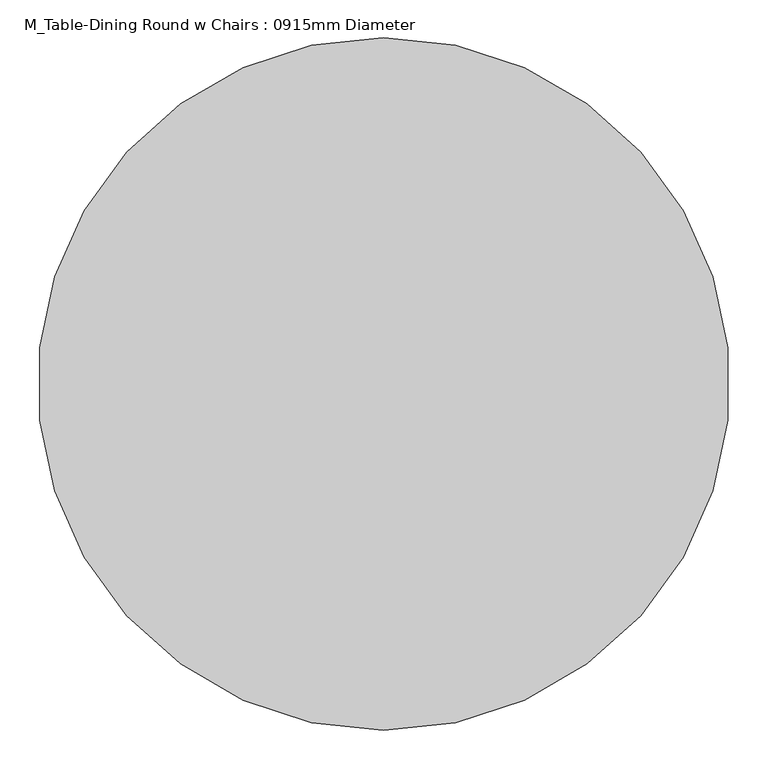
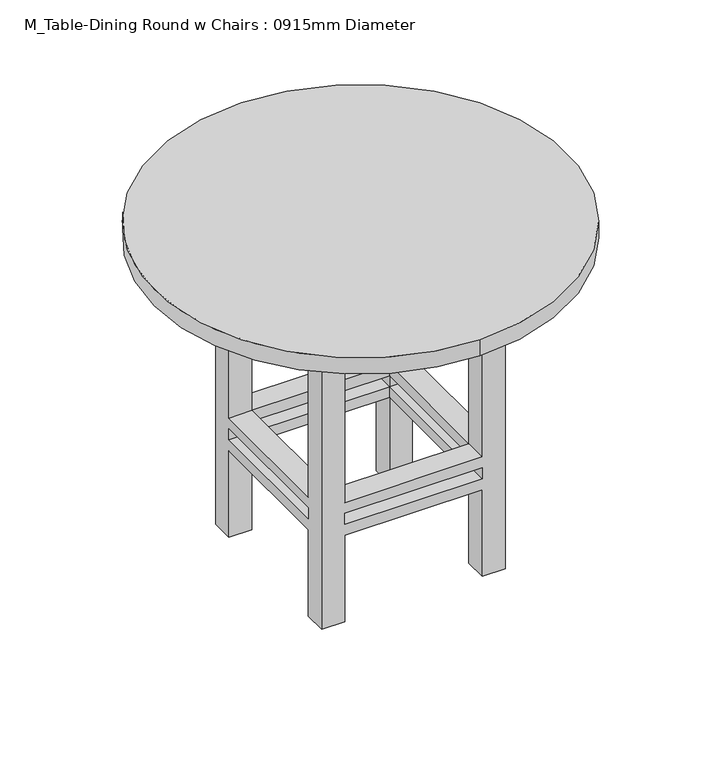
"""IFC4 building model written with IfcOpenShell, lengths in millimetres: furniture geometry, M_Table-Dining Round w Chairs : 0915mm Diameter."""

from ifc_helpers import new_model, si_unit, point, frame, frame_2d, origin, place, context, project, spatial, polyline, circle_curve, trimmed, segment, composite_curve, outline, extrude, faceted_brep, source, transform, mapped, element, save


def m_table_dining_round_w_chairs_0915mm_diameter_5defa876(model_context):
    return source(origin(), model_context, "Body", "SolidModel", [
        faceted_brep([(-48.8680328, 18.4713115, 647.7), (-99.6680328, 18.4713115, 647.7), (-99.6680328, -32.3286885, 647.7), (-48.8680328, -32.3286885, 647.7), (256.2319672, 18.4713115, 647.7), (256.2319672, -32.3286885, 647.7), (307.0319672, -32.3286885, 647.7), (307.0319672, 18.4713115, 647.7), (256.2319672, -388.2286885, 647.7), (307.0319672, -388.2286885, 647.7), (307.0319672, -337.4286885, 647.7), (256.2319672, -337.4286885, 647.7), (-48.8680328, -388.2286885, 647.7), (-48.8680328, -337.4286885, 647.7), (-99.6680328, -337.4286885, 647.7), (-99.6680328, -388.2286885, 647.7), (-48.8680328, 18.4713115, 0.0), (-48.8680328, -32.3286885, 0.0), (-99.6680328, -32.3286885, 0.0), (-99.6680328, 18.4713115, 0.0), (256.2319672, 18.4713115, 0.0), (307.0319672, 18.4713115, 0.0), (307.0319672, -32.3286885, 0.0), (256.2319672, -32.3286885, 0.0), (256.2319672, -388.2286885, 0.0), (256.2319672, -337.4286885, 0.0), (307.0319672, -337.4286885, 0.0), (307.0319672, -388.2286885, 0.0), (-48.8680328, -388.2286885, 0.0), (-99.6680328, -388.2286885, 0.0), (-99.6680328, -337.4286885, 0.0), (-48.8680328, -337.4286885, 0.0), (-48.8680328, 18.4713115, 279.4), (256.2319672, 18.4713115, 279.4), (256.2319672, 18.4713115, 203.2), (-48.8680328, 18.4713115, 203.2), (256.2319672, 18.4713115, 228.6), (256.2319672, 18.4713115, 254.0), (-48.8680328, 18.4713115, 254.0), (-48.8680328, 18.4713115, 228.6), (-99.6680328, -32.3286885, 203.2), (-99.6680328, -337.4286885, 203.2), (-99.6680328, -337.4286885, 279.4), (-99.6680328, -32.3286885, 279.4), (-99.6680328, -32.3286885, 228.6), (-99.6680328, -32.3286885, 254.0), (-99.6680328, -337.4286885, 254.0), (-99.6680328, -337.4286885, 228.6), (-48.8680328, -32.3286885, 279.4), (-48.8680328, -32.3286885, 203.2), (-48.8680328, -32.3286885, 228.6), (-48.8680328, -32.3286885, 254.0), (256.2319672, -32.3286885, 279.4), (256.2319672, -32.3286885, 203.2), (256.2319672, -32.3286885, 228.6), (256.2319672, -32.3286885, 254.0), (307.0319672, -32.3286885, 279.4), (307.0319672, -32.3286885, 203.2), (307.0319672, -32.3286885, 228.6), (307.0319672, -32.3286885, 254.0), (307.0319672, -337.4286885, 279.4), (307.0319672, -337.4286885, 203.2), (307.0319672, -337.4286885, 228.6), (307.0319672, -337.4286885, 254.0), (256.2319672, -388.2286885, 279.4), (-48.8680328, -388.2286885, 279.4), (-48.8680328, -388.2286885, 203.2), (256.2319672, -388.2286885, 203.2), (-48.8680328, -388.2286885, 228.6), (-48.8680328, -388.2286885, 254.0), (256.2319672, -388.2286885, 254.0), (256.2319672, -388.2286885, 228.6), (256.2319672, -337.4286885, 279.4), (256.2319672, -337.4286885, 203.2), (256.2319672, -337.4286885, 228.6), (256.2319672, -337.4286885, 254.0), (-48.8680328, -337.4286885, 279.4), (-48.8680328, -337.4286885, 203.2), (-48.8680328, -337.4286885, 228.6), (-48.8680328, -337.4286885, 254.0)], [[[0, 1, 2, 3]], [[4, 5, 6, 7]], [[8, 9, 10, 11]], [[12, 13, 14, 15]], [[16, 17, 18, 19]], [[20, 21, 22, 23]], [[24, 25, 26, 27]], [[28, 29, 30, 31]], [[1, 0, 32, 33, 4, 7, 21, 20, 34, 35, 16, 19], [36, 37, 38, 39]], [[2, 1, 19, 18, 40, 41, 30, 29, 15, 14, 42, 43], [44, 45, 46, 47]], [[3, 2, 43, 48]], [[18, 17, 49, 40]], [[44, 50, 51, 45]], [[0, 3, 48, 32]], [[17, 16, 35, 49]], [[50, 39, 38, 51]], [[5, 4, 33, 52]], [[20, 23, 53, 34]], [[36, 54, 55, 37]], [[6, 5, 52, 56]], [[23, 22, 57, 53]], [[54, 58, 59, 55]], [[21, 7, 6, 56, 60, 10, 9, 27, 26, 61, 57, 22], [62, 63, 59, 58]], [[27, 9, 8, 64, 65, 12, 15, 29, 28, 66, 67, 24], [68, 69, 70, 71]], [[11, 10, 60, 72]], [[26, 25, 73, 61]], [[62, 74, 75, 63]], [[8, 11, 72, 64]], [[25, 24, 67, 73]], [[74, 71, 70, 75]], [[13, 12, 65, 76]], [[28, 31, 77, 66]], [[68, 78, 79, 69]], [[14, 13, 76, 42]], [[31, 30, 41, 77]], [[78, 47, 46, 79]], [[54, 74, 62, 58]], [[74, 78, 68, 71]], [[78, 50, 44, 47]], [[50, 54, 36, 39]], [[53, 49, 35, 34]], [[49, 77, 41, 40]], [[77, 73, 67, 66]], [[73, 53, 57, 61]], [[74, 54, 53, 73]], [[78, 74, 73, 77]], [[50, 78, 77, 49]], [[54, 50, 49, 53]], [[52, 72, 60, 56]], [[72, 76, 65, 64]], [[76, 48, 43, 42]], [[48, 52, 33, 32]], [[55, 51, 38, 37]], [[51, 79, 46, 45]], [[79, 75, 70, 69]], [[75, 55, 59, 63]], [[72, 52, 55, 75]], [[76, 72, 75, 79]], [[48, 76, 79, 51]], [[52, 48, 51, 55]]]),
        extrude(outline(polyline([(332.4319672, 43.8713115), (332.4319672, -413.6286885), (-125.0680328, -413.6286885), (-125.0680328, 43.8713115), (332.4319672, 43.8713115)]), holes=[polyline([(307.0319672, 18.4713115), (-99.6680328, 18.4713115), (-99.6680328, -388.2286885), (307.0319672, -388.2286885), (307.0319672, 18.4713115)])]), frame((0.0, 0.0, 647.7), z_axis=(0.0, 0.0, 1.0), x_axis=(1.0, 0.0, 0.0)), (0.0, 0.0, 1.0), 76.2),
        extrude(outline(composite_curve([segment(trimmed(circle_curve(frame_2d((103.6819672, -184.8786885)), 457.5), [point((103.6819672, -642.3786885))], [point((103.6819672, 272.6213115))], False, "CARTESIAN"), True, "CONTINUOUS"), segment(trimmed(circle_curve(frame_2d((103.6819672, -184.8786885)), 457.5), [point((103.6819672, 272.6213115))], [point((103.6819672, -642.3786885))], False, "CARTESIAN"), True, "CONTINUOUS")], self_intersect=False)), frame((0.0, 0.0, 723.9), z_axis=(0.0, 0.0, 1.0), x_axis=(1.0, 0.0, 0.0)), (0.0, 0.0, 1.0), 38.1),
    ])


if __name__ == "__main__":
    model = new_model("IFC4")
    model_context = context("Model", 3, world=origin())
    ifc_project = project(units=[si_unit("LENGTHUNIT", "METRE", prefix="MILLI")], contexts=[model_context])
    site = spatial("IfcSite", under=ifc_project)
    building = spatial("IfcBuilding", under=site)
    placement = place(None, origin())
    m_table_dining_round_w_chairs_0915mm_diameter_shape = m_table_dining_round_w_chairs_0915mm_diameter_5defa876(model_context)
    element("IfcFurniture", 1, ObjectType="M_Table-Dining Round w Chairs : 0915mm Diameter", at=placement, inside=building, context=model_context, shape_type="MappedRepresentation", body=[
        mapped(m_table_dining_round_w_chairs_0915mm_diameter_shape, transform((0.0, 0.0, 0.0), x_axis=(1.0, 0.0, 0.0), y_axis=(0.0, 1.0, 0.0), z_axis=(0.0, 0.0, 1.0))),
    ])
    save(model, "model.ifc")

# Revit data of these elements
# Type "M_Table-Dining Round w Chairs : 0915mm Diameter"
#   Radius = 1' - 6.01181"
#   Diameter = 3' - 0.02362"
#   Height = 2' - 6"
#   Chairs = 4
#   Base Material = Pine
#   Top Material = Laminate, Linen, Matte
#   Default Elevation = 0
# Element 1 (IfcFurniture, "M_Table-Dining Round w Chairs : 0915mm Diameter")
#   Materials on its faces: "Pine", "Laminate, Linen, Matte"
# Materials
#   "Pine": class "Wood", colour RGB 223 192 134, transparency 0, Description = "Pinus Echinata", Cost = 0
#   "Laminate, Linen, Matte": class "Plastic", colour RGB 249 239 230, transparency 0, Description = "Plastic Laminate - Linen, Matte", Cost = 0
